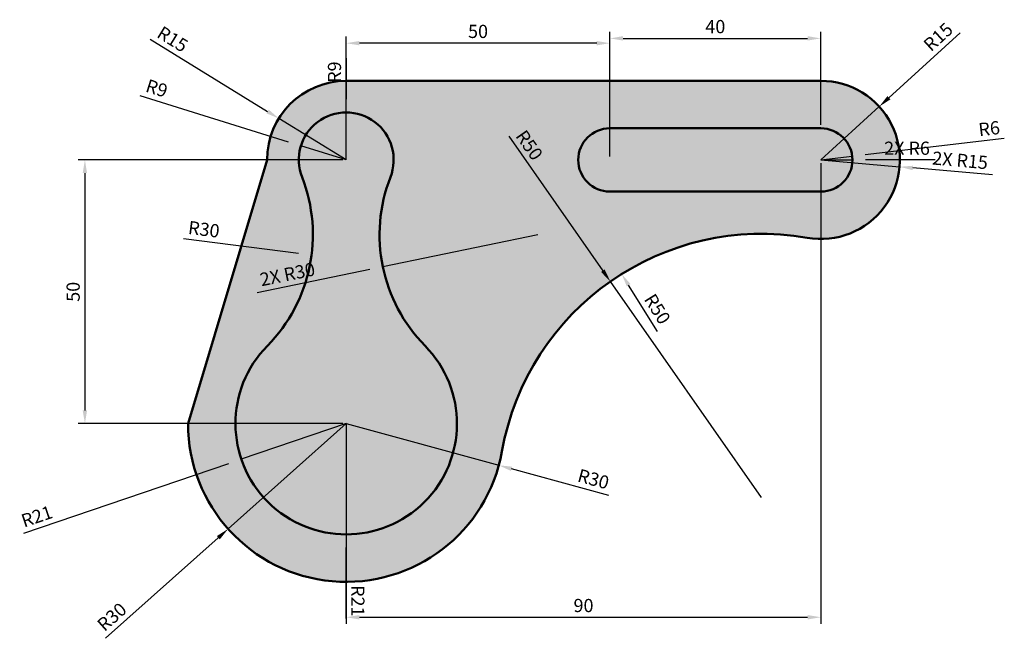
# Model space of a CAD drawing. Units: millimetres. Extents: x 2487 to 2673, y 1324 to 1441.
import ezdxf

# ---------------------------------------------------------------- set-up
doc = ezdxf.new("R2010")
doc.units = ezdxf.units.MM
for name, color, linetype, lineweight in [('M-DIMS', 2, 'Continuous', 25), ('M-HATC', 8, 'Continuous', 18), ('M-OUTL', 7, 'Continuous', 50)]:
    doc.layers.add(name, color=color, linetype=linetype, lineweight=lineweight)
doc.styles.get("Standard").update_dxf_attribs({"font": 'arial.ttf'})
doc.dimstyles.new('ISO-25', dxfattribs={"dimtxt": 2.5, "dimasz": 2.5, "dimexe": 1.25, "dimexo": 0.625, "dimtad": 1, "dimtxsty": 'Standard', "dimcen": 2.5, "dimadec": 0, "dimazin": 0, "dimtfac": 1, "dimtmove": 0, "dimatfit": 3, "dimfxl": 1, "dimarcsym": 0})

# ---------------------------------------------------------------- blocks, each defined once
blk = doc.blocks.new('*D1')
at = {"layer": 'Defpoints', "color": 0, "transparency": 16777216}
for p in [(2638.48, 1437.75), (2598.48, 1420.7), (2638.48, 1420.7)]:
    blk.add_point(p, dxfattribs=at)
at = {"layer": 'M-DIMS', "color": 0, "lineweight": -2, "transparency": 16777216}
for p, q in [((2598.48, 1421.33), (2598.48, 1439)), ((2600.98, 1437.75), (2635.98, 1437.75)), ((2638.48, 1421.33), (2638.48, 1439))]:
    blk.add_line(p, q, dxfattribs=at)
at = {"layer": 'M-DIMS', "color": 0, "transparency": 16777216}
for points in [[(2600.98, 1438.17), (2600.98, 1437.34), (2598.48, 1437.75)], [(2635.98, 1438.17), (2635.98, 1437.34), (2638.48, 1437.75)]]:
    blk.add_solid(points, dxfattribs=at)
at = {"layer": 'M-DIMS', "color": 0, "transparency": 16777216, "insert": (2618.48, 1439.66), "char_height": 2.5, "attachment_point": 5}
blk.add_mtext('40', dxfattribs=at)
blk = doc.blocks.new('*D2')
at = {"layer": 'Defpoints', "color": 0, "transparency": 16777216}
for p in [(2548.48, 1436.84), (2548.48, 1414.7), (2598.48, 1414.7)]:
    blk.add_point(p, dxfattribs=at)
at = {"layer": 'M-DIMS', "color": 0, "lineweight": -2, "transparency": 16777216}
for p, q in [((2548.48, 1415.33), (2548.48, 1438.09)), ((2598.48, 1415.33), (2598.48, 1438.09)), ((2595.98, 1436.84), (2550.98, 1436.84))]:
    blk.add_line(p, q, dxfattribs=at)
at = {"layer": 'M-DIMS', "color": 0, "transparency": 16777216}
for points in [[(2550.98, 1437.26), (2550.98, 1436.43), (2548.48, 1436.84)], [(2595.98, 1437.26), (2595.98, 1436.43), (2598.48, 1436.84)]]:
    blk.add_solid(points, dxfattribs=at)
at = {"layer": 'M-DIMS', "color": 0, "transparency": 16777216, "insert": (2573.48, 1438.75), "char_height": 2.5, "attachment_point": 5}
blk.add_mtext('50', dxfattribs=at)
blk = doc.blocks.new('*D3')
at = {"layer": 'Defpoints', "color": 0, "transparency": 16777216}
for p in [(2548.48, 1414.7), (2498.93, 1364.7), (2548.48, 1364.7)]:
    blk.add_point(p, dxfattribs=at)
at = {"layer": 'M-DIMS', "color": 0, "lineweight": -2, "transparency": 16777216}
for p, q in [((2547.85, 1414.7), (2497.68, 1414.7)), ((2498.93, 1412.2), (2498.93, 1367.2)), ((2547.85, 1364.7), (2497.68, 1364.7))]:
    blk.add_line(p, q, dxfattribs=at)
at = {"layer": 'M-DIMS', "color": 0, "transparency": 16777216}
for points in [[(2498.51, 1412.2), (2499.34, 1412.2), (2498.93, 1414.7)], [(2498.51, 1367.2), (2499.34, 1367.2), (2498.93, 1364.7)]]:
    blk.add_solid(points, dxfattribs=at)
at = {"layer": 'M-DIMS', "color": 0, "transparency": 16777216, "insert": (2497.02, 1389.7), "char_height": 2.5, "attachment_point": 5, "rotation": 90}
blk.add_mtext('50', dxfattribs=at)
blk = doc.blocks.new('*D4')
at = {"layer": 'Defpoints', "color": 0, "transparency": 16777216}
for p in [(2638.48, 1414.7), (2548.48, 1364.7), (2638.48, 1327.99)]:
    blk.add_point(p, dxfattribs=at)
at = {"layer": 'M-DIMS', "color": 0, "lineweight": -2, "transparency": 16777216}
for p, q in [((2638.48, 1414.08), (2638.48, 1326.74)), ((2548.48, 1364.08), (2548.48, 1326.74)), ((2550.98, 1327.99), (2635.98, 1327.99))]:
    blk.add_line(p, q, dxfattribs=at)
at = {"layer": 'M-DIMS', "color": 0, "transparency": 16777216}
for points in [[(2550.98, 1328.4), (2550.98, 1327.57), (2548.48, 1327.99)], [(2635.98, 1328.4), (2635.98, 1327.57), (2638.48, 1327.99)]]:
    blk.add_solid(points, dxfattribs=at)
at = {"layer": 'M-DIMS', "color": 0, "transparency": 16777216, "insert": (2593.48, 1329.89), "char_height": 2.5, "attachment_point": 5}
blk.add_mtext('90', dxfattribs=at)
blk = doc.blocks.new('*D5')
at = {"layer": 'Defpoints', "color": 0, "transparency": 16777216}
for p in [(2644.44, 1415.4), (2638.48, 1414.7)]:
    blk.add_point(p, dxfattribs=at)
at = {"layer": 'M-DIMS', "color": 0, "lineweight": -2, "transparency": 16777216}
for p, q in [((2673.28, 1418.74), (2646.92, 1415.68)), ((2638.48, 1414.7), (2644.44, 1415.4))]:
    blk.add_line(p, q, dxfattribs=at)
at = {"layer": 'M-DIMS', "color": 0, "transparency": 16777216}
blk.add_solid([(2646.87, 1416.1), (2646.97, 1415.27), (2644.44, 1415.4)], dxfattribs=at)
at = {"layer": 'M-DIMS', "color": 0, "transparency": 16777216, "insert": (2670.44, 1420.33), "char_height": 2.5, "attachment_point": 5, "rotation": 6.616}
blk.add_mtext('R6', dxfattribs=at)
blk = doc.blocks.new('*D6')
at = {"layer": 'Defpoints', "color": 0, "transparency": 16777216}
for p in [(2539.89, 1417.39), (2548.48, 1414.7)]:
    blk.add_point(p, dxfattribs=at)
at = {"layer": 'M-DIMS', "color": 0, "lineweight": -2, "transparency": 16777216}
for p, q in [((2509.37, 1426.95), (2537.5, 1418.14)), ((2548.48, 1414.7), (2539.89, 1417.39))]:
    blk.add_line(p, q, dxfattribs=at)
at = {"layer": 'M-DIMS', "color": 0, "transparency": 16777216}
blk.add_solid([(2537.63, 1418.54), (2537.38, 1417.74), (2539.89, 1417.39)], dxfattribs=at)
at = {"layer": 'M-DIMS', "color": 0, "transparency": 16777216, "insert": (2512.46, 1427.98), "char_height": 2.5, "attachment_point": 5, "rotation": 342.6094}
blk.add_mtext('R9', dxfattribs=at)
blk = doc.blocks.new('*D7')
at = {"layer": 'Defpoints', "color": 0, "transparency": 16777216}
for p in [(2548.48, 1364.7), (2528.59, 1357.96)]:
    blk.add_point(p, dxfattribs=at)
at = {"layer": 'M-DIMS', "color": 0, "lineweight": -2, "transparency": 16777216}
for p, q in [((2548.48, 1364.7), (2528.59, 1357.96)), ((2487.32, 1343.95), (2526.23, 1357.15))]:
    blk.add_line(p, q, dxfattribs=at)
at = {"layer": 'M-DIMS', "color": 0, "transparency": 16777216}
blk.add_solid([(2526.09, 1357.55), (2526.36, 1356.76), (2528.59, 1357.96)], dxfattribs=at)
at = {"layer": 'M-DIMS', "color": 0, "transparency": 16777216, "insert": (2489.91, 1346.81), "char_height": 2.5, "attachment_point": 5, "rotation": 18.7456}
blk.add_mtext('R21', dxfattribs=at)
blk = doc.blocks.new('*D8')
at = {"layer": 'Defpoints', "color": 0, "transparency": 16777216}
for p in [(2600.72, 1393.07), (2627.24, 1350.68)]:
    blk.add_point(p, dxfattribs=at)
at = {"layer": 'M-DIMS', "color": 0, "lineweight": -2, "transparency": 16777216}
blk.add_line((2607.52, 1382.2), (2602.04, 1390.95), dxfattribs=at)
at = {"layer": 'M-DIMS', "color": 0, "transparency": 16777216}
blk.add_solid([(2602.4, 1391.17), (2601.69, 1390.73), (2600.72, 1393.07)], dxfattribs=at)
at = {"layer": 'M-DIMS', "color": 0, "transparency": 16777216, "insert": (2607.22, 1386.27), "char_height": 2.5, "attachment_point": 5, "rotation": 302.0383}
blk.add_mtext('R50', dxfattribs=at)
blk = doc.blocks.new('*D9')
at = {"layer": 'Defpoints', "color": 0, "transparency": 16777216}
for p in [(2548.48, 1364.7), (2526.09, 1344.74)]:
    blk.add_point(p, dxfattribs=at)
at = {"layer": 'M-DIMS', "color": 0, "lineweight": -2, "transparency": 16777216}
for p, q in [((2548.48, 1364.7), (2526.09, 1344.74)), ((2502.83, 1324), (2524.22, 1343.07))]:
    blk.add_line(p, q, dxfattribs=at)
at = {"layer": 'M-DIMS', "color": 0, "transparency": 16777216}
blk.add_solid([(2523.95, 1343.38), (2524.5, 1342.76), (2526.09, 1344.74)], dxfattribs=at)
at = {"layer": 'M-DIMS', "color": 0, "transparency": 16777216, "insert": (2504.26, 1327.82), "char_height": 2.5, "attachment_point": 5, "rotation": 41.7263}
blk.add_mtext('R30', dxfattribs=at)
blk = doc.blocks.new('*D10')
at = {"layer": 'Defpoints', "color": 0, "transparency": 16777216}
for p in [(2649.56, 1424.82), (2638.48, 1414.7)]:
    blk.add_point(p, dxfattribs=at)
at = {"layer": 'M-DIMS', "color": 0, "lineweight": -2, "transparency": 16777216}
for p, q in [((2664.92, 1438.83), (2651.4, 1426.5)), ((2638.48, 1414.7), (2649.56, 1424.82))]:
    blk.add_line(p, q, dxfattribs=at)
at = {"layer": 'M-DIMS', "color": 0, "transparency": 16777216}
blk.add_solid([(2651.12, 1426.81), (2651.69, 1426.19), (2649.56, 1424.82)], dxfattribs=at)
at = {"layer": 'M-DIMS', "color": 0, "transparency": 16777216, "insert": (2660.96, 1437.79), "char_height": 2.5, "attachment_point": 5, "rotation": 42.3833}
blk.add_mtext('R15', dxfattribs=at)
blk = doc.blocks.new('*D11')
at = {"layer": 'Defpoints', "color": 0, "transparency": 16777216}
for p in [(2535.71, 1422.57), (2548.48, 1414.7)]:
    blk.add_point(p, dxfattribs=at)
at = {"layer": 'M-DIMS', "color": 0, "lineweight": -2, "transparency": 16777216}
for p, q in [((2511.31, 1437.61), (2533.58, 1423.89)), ((2548.48, 1414.7), (2535.71, 1422.57))]:
    blk.add_line(p, q, dxfattribs=at)
at = {"layer": 'M-DIMS', "color": 0, "transparency": 16777216}
blk.add_solid([(2533.8, 1424.24), (2533.36, 1423.53), (2535.71, 1422.57)], dxfattribs=at)
at = {"layer": 'M-DIMS', "color": 0, "transparency": 16777216, "insert": (2515.39, 1437.33), "char_height": 2.5, "attachment_point": 5, "rotation": 328.3577}
blk.add_mtext('R15', dxfattribs=at)
blk = doc.blocks.new('*D12')
at = {"layer": 'Defpoints', "color": 0, "transparency": 16777216}
for p in [(2512.16, 1400.5), (2541.91, 1396.7)]:
    blk.add_point(p, dxfattribs=at)
at = {"layer": 'M-DIMS', "color": 0, "lineweight": -2, "transparency": 16777216}
blk.add_line((2517.64, 1399.8), (2539.43, 1397.02), dxfattribs=at)
at = {"layer": 'M-DIMS', "color": 0, "transparency": 16777216}
blk.add_solid([(2539.49, 1397.43), (2539.38, 1396.61), (2541.91, 1396.7)], dxfattribs=at)
at = {"layer": 'M-DIMS', "color": 0, "transparency": 16777216, "insert": (2521.46, 1401.23), "char_height": 2.5, "attachment_point": 5, "rotation": 352.7204}
blk.add_mtext('R30', dxfattribs=at)
blk = doc.blocks.new('*D13')
at = {"layer": 'Defpoints', "color": 0, "transparency": 16777216}
for p in [(2598.58, 1391.65), (2627.24, 1350.68)]:
    blk.add_point(p, dxfattribs=at)
at = {"layer": 'M-DIMS', "color": 0, "lineweight": -2, "transparency": 16777216}
for p, q in [((2579.31, 1419.19), (2597.15, 1393.7)), ((2627.24, 1350.68), (2598.58, 1391.65))]:
    blk.add_line(p, q, dxfattribs=at)
at = {"layer": 'M-DIMS', "color": 0, "transparency": 16777216}
blk.add_solid([(2597.49, 1393.94), (2596.8, 1393.46), (2598.58, 1391.65)], dxfattribs=at)
at = {"layer": 'M-DIMS', "color": 0, "transparency": 16777216, "insert": (2582.94, 1417.32), "char_height": 2.5, "attachment_point": 5, "rotation": 304.9755}
blk.add_mtext('R50', dxfattribs=at)
blk = doc.blocks.new('*D14')
at = {"layer": 'Defpoints', "color": 0, "transparency": 16777216}
for p in [(2584.8, 1400.5), (2555.42, 1394.46)]:
    blk.add_point(p, dxfattribs=at)
at = {"layer": 'M-DIMS', "color": 0, "lineweight": -2, "transparency": 16777216}
for p, q in [((2584.8, 1400.5), (2555.42, 1394.46)), ((2531.6, 1389.57), (2552.97, 1393.96))]:
    blk.add_line(p, q, dxfattribs=at)
at = {"layer": 'M-DIMS', "color": 0, "transparency": 16777216}
blk.add_solid([(2552.88, 1394.37), (2553.05, 1393.55), (2555.42, 1394.46)], dxfattribs=at)
at = {"layer": 'M-DIMS', "color": 0, "transparency": 16777216, "insert": (2537.4, 1392.7), "char_height": 2.5, "attachment_point": 5, "rotation": 11.6157}
blk.add_mtext('2X R30', dxfattribs=at)
blk = doc.blocks.new('*D15')
at = {"layer": 'Defpoints', "color": 0, "transparency": 16777216}
for p in [(2548.48, 1364.7), (2577.42, 1356.8)]:
    blk.add_point(p, dxfattribs=at)
at = {"layer": 'M-DIMS', "color": 0, "lineweight": -2, "transparency": 16777216}
for p, q in [((2548.48, 1364.7), (2577.42, 1356.8)), ((2598.26, 1351.1), (2579.83, 1356.14))]:
    blk.add_line(p, q, dxfattribs=at)
at = {"layer": 'M-DIMS', "color": 0, "transparency": 16777216}
blk.add_solid([(2579.94, 1356.54), (2579.72, 1355.73), (2577.42, 1356.8)], dxfattribs=at)
at = {"layer": 'M-DIMS', "color": 0, "transparency": 16777216, "insert": (2595.28, 1353.88), "char_height": 2.5, "attachment_point": 5, "rotation": 344.7141}
blk.add_mtext('R30', dxfattribs=at)
blk = doc.blocks.new('*D16')
at = {"layer": 'Defpoints', "color": 0, "transparency": 16777216}
for p in [(2548.48, 1364.7), (2548.48, 1343.7)]:
    blk.add_point(p, dxfattribs=at)
at = {"layer": 'M-DIMS', "color": 0, "lineweight": -2, "transparency": 16777216}
for p, q in [((2548.48, 1364.7), (2548.48, 1343.7)), ((2548.48, 1327.73), (2548.48, 1341.2))]:
    blk.add_line(p, q, dxfattribs=at)
at = {"layer": 'M-DIMS', "color": 0, "transparency": 16777216}
blk.add_solid([(2548.9, 1341.2), (2548.06, 1341.2), (2548.48, 1343.7)], dxfattribs=at)
at = {"layer": 'M-DIMS', "color": 0, "transparency": 16777216, "insert": (2550.36, 1331.1), "char_height": 2.5, "attachment_point": 5, "rotation": 270.0013}
blk.add_mtext('R21', dxfattribs=at)
blk = doc.blocks.new('*D17')
at = {"layer": 'Defpoints', "color": 0, "transparency": 16777216}
for p in [(2638.48, 1414.7), (2653.42, 1413.4)]:
    blk.add_point(p, dxfattribs=at)
at = {"layer": 'M-DIMS', "color": 0, "lineweight": -2, "transparency": 16777216}
for p, q in [((2638.48, 1414.7), (2653.42, 1413.4)), ((2671.01, 1411.87), (2655.91, 1413.19))]:
    blk.add_line(p, q, dxfattribs=at)
at = {"layer": 'M-DIMS', "color": 0, "transparency": 16777216}
blk.add_solid([(2655.95, 1413.6), (2655.88, 1412.77), (2653.42, 1413.4)], dxfattribs=at)
at = {"layer": 'M-DIMS', "color": 0, "transparency": 16777216, "insert": (2664.87, 1414.31), "char_height": 2.5, "attachment_point": 5, "rotation": 355.0229}
blk.add_mtext('2X R15', dxfattribs=at)
blk = doc.blocks.new('*D18')
at = {"layer": 'Defpoints', "color": 0, "transparency": 16777216}
for p in [(2548.48, 1423.7), (2548.48, 1414.7)]:
    blk.add_point(p, dxfattribs=at)
at = {"layer": 'M-DIMS', "color": 0, "lineweight": -2, "transparency": 16777216}
for p, q in [((2548.48, 1433.99), (2548.48, 1426.2)), ((2548.48, 1414.7), (2548.48, 1423.7))]:
    blk.add_line(p, q, dxfattribs=at)
at = {"layer": 'M-DIMS', "color": 0, "transparency": 16777216}
blk.add_solid([(2548.06, 1426.2), (2548.9, 1426.2), (2548.48, 1423.7)], dxfattribs=at)
at = {"layer": 'M-DIMS', "color": 0, "transparency": 16777216, "insert": (2546.58, 1431.35), "char_height": 2.5, "attachment_point": 5, "rotation": 89.9969}
blk.add_mtext('R9', dxfattribs=at)
blk = doc.blocks.new('*D19')
at = {"layer": 'Defpoints', "color": 0, "transparency": 16777216}
for p in [(2638.48, 1414.7), (2644.48, 1414.7)]:
    blk.add_point(p, dxfattribs=at)
at = {"layer": 'M-DIMS', "color": 0, "lineweight": -2, "transparency": 16777216}
for p, q in [((2638.48, 1414.7), (2644.48, 1414.7)), ((2660.17, 1414.7), (2646.98, 1414.7))]:
    blk.add_line(p, q, dxfattribs=at)
at = {"layer": 'M-DIMS', "color": 0, "transparency": 16777216}
blk.add_solid([(2646.98, 1415.12), (2646.98, 1414.29), (2644.48, 1414.7)], dxfattribs=at)
at = {"layer": 'M-DIMS', "color": 0, "transparency": 16777216, "insert": (2654.83, 1416.6), "char_height": 2.5, "attachment_point": 5, "rotation": 359.9965}
blk.add_mtext('2X R6', dxfattribs=at)

msp = doc.modelspace()

# ---------------------------------------------------------------- hatches: boundary and pattern name
at = {"layer": 'M-HATC'}
h = msp.add_hatch(color=256, dxfattribs=at)
h.dxf.hatch_style = 1
h.set_gradient(color1=(0, 0, 255), color2=(255, 255, 0), tint=1)
h.paths.add_polyline_path([(2638.479, 1429.704), (2548.479, 1429.704, 0.4142136), (2533.479, 1414.704), (2518.479, 1364.704, 0.9155769), (2578.014, 1359.446, -0.4135097), (2635.885, 1399.93, 1.0908906)])
h.paths.add_polyline_path([(2556.861, 1411.427, 0.295914), (2563.435, 1379.446, -2.3896708), (2533.522, 1379.446, 0.295914), (2540.096, 1411.427, -1.4646369)], flags=16)
h.paths.add_polyline_path([(2598.479, 1420.704), (2638.479, 1420.704, -1), (2638.479, 1408.704), (2598.479, 1408.704, -1)], flags=16)
h = msp.add_hatch(color=256, dxfattribs=at)
h.dxf.hatch_style = 1
h.set_gradient(color1=(255, 0, 0), tint=1)
h.paths.add_polyline_path([(2638.479, 1420.704), (2598.479, 1420.704, 1), (2598.479, 1408.704), (2638.479, 1408.704, 1)])
h.paths.add_polyline_path([(2556.861, 1411.427, 1.4646369), (2540.096, 1411.427, -0.295914), (2533.522, 1379.446, 2.3896708), (2563.435, 1379.446, -0.295914)])

# ---------------------------------------------------------------- linework, layer by layer
at = {"layer": 'M-OUTL'}
for p, q in [((2548.479, 1429.704), (2638.479, 1429.704)), ((2598.479, 1420.704), (2638.479, 1420.704)), ((2533.479, 1414.704), (2518.479, 1364.704)), ((2598.479, 1408.704), (2638.479, 1408.704))]:
    msp.add_line(p, q, dxfattribs=at)
for centre, radius, start, end in [((2548.479, 1414.704), 15, 90, 180), ((2638.479, 1414.704), 15, 260.04372, 90), ((2548.479, 1414.704), 9, 338.64764, 201.35236), ((2598.479, 1414.704), 6, 90, 270), ((2638.479, 1414.704), 6, 270, 90), ((2512.156, 1400.504), 30, 315.41547, 21.35236), ((2584.802, 1400.504), 30, 158.64764, 224.58453), ((2627.24, 1350.683), 50, 80.04372, 169.90599), ((2548.479, 1364.704), 21, 135.41547, 44.58453), ((2548.479, 1364.704), 30, 180, 349.90599)]:
    msp.add_arc(centre, radius, start, end, dxfattribs=at)

# ---------------------------------------------------------------- dimensions: what is measured, and where the dimension line sits
at = {"layer": 'M-DIMS'}
for center, mpoint, override, picture, middle in [((2548.479, 1414.704), (2535.708, 1422.574), {"dimclrd": 0, "dimclre": 0, "dimclrt": 0}, '*D11', (2514.393, 1435.709)), ((2638.479, 1414.704), (2649.558, 1424.816), {"dimclrd": 0, "dimclre": 0, "dimclrt": 0}, '*D10', (2662.242, 1436.39)), ((2548.479, 1414.704), (2539.89, 1417.394), {"dimclrd": 0, "dimclre": 0, "dimclrt": 0}, '*D6', (2511.891, 1426.164)), ((2638.479, 1414.704), (2644.439, 1415.396), {"dimclrd": 0, "dimclre": 0, "dimclrt": 0}, '*D5', (2670.658, 1418.437)), ((2627.24, 1350.683), (2598.579, 1391.653), {"dimdec": 0, "dimlfac": 1, "dimrnd": 0, "dimzin": 0, "dimdsep": 46, "dimlunit": 2}, '*D13', (2581.382, 1416.235)), ((2512.156, 1400.504), (2541.914, 1396.703), {"dimclrd": 0, "dimclre": 0, "dimclrt": 0}, '*D12', (2521.217, 1399.347)), ((2627.24, 1350.683), (2600.716, 1393.068), {"dimclrd": 0, "dimclre": 0, "dimclrt": 0}, '*D8', (2605.604, 1385.257)), ((2548.479, 1364.704), (2528.592, 1357.956), {"dimclrd": 0, "dimclre": 0, "dimclrt": 0}, '*D7', (2490.51, 1345.032)), ((2548.479, 1364.704), (2526.089, 1344.737), {"dimclrd": 0, "dimclre": 0, "dimclrt": 0}, '*D9', (2505.522, 1326.396)), ((2548.479, 1364.704), (2548.479, 1343.704), {"dimdec": 0, "dimlfac": 1, "dimrnd": 0, "dimzin": 0, "dimdsep": 46, "dimlunit": 2}, '*D16', (2548.479, 1331.104)), ((2548.479, 1364.704), (2577.417, 1356.795), {"dimdec": 0, "dimlfac": 1, "dimrnd": 0, "dimzin": 0, "dimdsep": 46, "dimlunit": 2}, '*D15', (2594.78, 1352.05))]:
    dim = msp.add_radius_dim(center=center, mpoint=mpoint, dimstyle='ISO-25', override=override, dxfattribs=at)
    dim.commit()
    dim.dimension.update_dxf_attribs({"geometry": picture, "text_midpoint": middle, "dimtype": 164})
for base, p1, p2, picture, middle in [((2548.479, 1436.845), (2598.479, 1414.704), (2548.479, 1414.704), '*D2', (2573.479, 1438.746)), ((2638.479, 1437.754), (2598.479, 1420.704), (2638.479, 1420.704), '*D1', (2618.479, 1439.655)), ((2638.479, 1327.987), (2548.479, 1364.704), (2638.479, 1414.704), '*D4', (2593.479, 1329.889))]:
    dim = msp.add_linear_dim(base=base, p1=p1, p2=p2, dimstyle='ISO-25', override={"dimclrd": 0, "dimclre": 0, "dimclrt": 0}, dxfattribs=at)
    dim.commit()
    dim.dimension.update_dxf_attribs({"geometry": picture, "text_midpoint": middle})
dim = msp.add_radius_dim(center=(2548.479, 1414.704), mpoint=(2548.479, 1423.704), dimstyle='ISO-25', override={"dimdec": 0, "dimlfac": 1, "dimrnd": 0, "dimzin": 0, "dimdsep": 46, "dimlunit": 2}, dxfattribs=at)
dim.commit()
dim.dimension.update_dxf_attribs({"geometry": '*D18', "text_midpoint": (2546.578, 1431.348)})
for mpoint, picture, middle in [((2644.479, 1414.704), '*D19', (2654.826, 1416.605)), ((2653.422, 1413.403), '*D17', (2664.873, 1414.314))]:
    dim = msp.add_radius_dim(center=(2638.479, 1414.704), mpoint=mpoint, text='2X <>', dimstyle='ISO-25', override={"dimdec": 0, "dimlfac": 1, "dimrnd": 0, "dimzin": 0, "dimdsep": 46, "dimlunit": 2}, dxfattribs=at)
    dim.commit()
    dim.dimension.update_dxf_attribs({"geometry": picture, "text_midpoint": middle})
dim = msp.add_linear_dim(base=(2498.926, 1364.704), p1=(2548.479, 1414.704), p2=(2548.479, 1364.704), angle=90, dimstyle='ISO-25', override={"dimclrd": 0, "dimclre": 0, "dimclrt": 0}, dxfattribs=at)
dim.commit()
dim.dimension.update_dxf_attribs({"geometry": '*D3', "text_midpoint": (2497.025, 1389.704)})
dim = msp.add_radius_dim(center=(2584.802, 1400.504), mpoint=(2555.416, 1394.464), text='2X <>', dimstyle='ISO-25', override={"dimdec": 0, "dimlfac": 1, "dimrnd": 0, "dimzin": 0, "dimdsep": 46, "dimlunit": 2}, dxfattribs=at)
dim.commit()
dim.dimension.update_dxf_attribs({"geometry": '*D14', "text_midpoint": (2537.785, 1390.84), "dimtype": 164})

doc.saveas('drawing.dxf')
